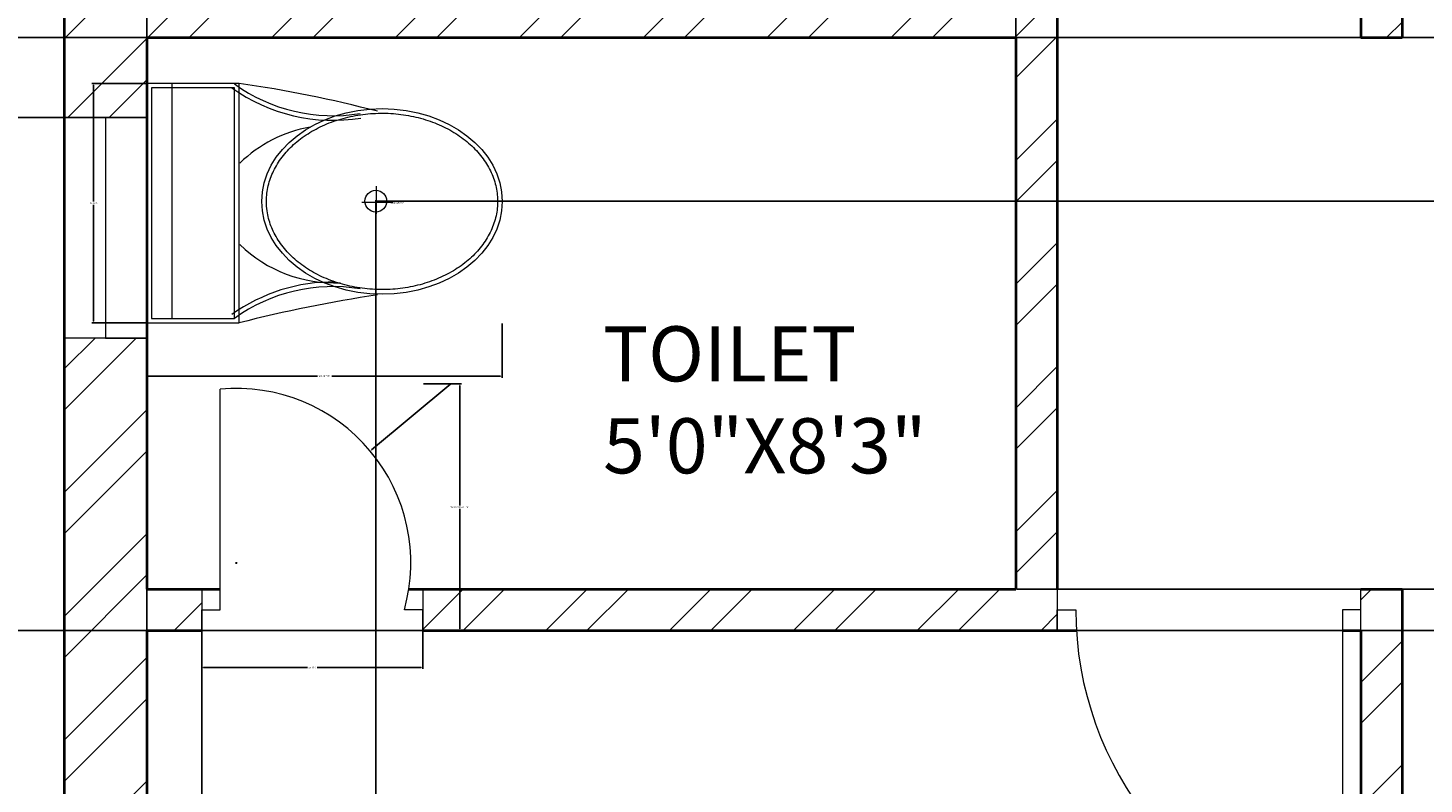
# Model space of a CAD drawing. Units: inches. Extents: x 1355 to 2746, y 1171 to 2751.
# Tile 8 of 24: x 1511 to 1663, y 1901 to 1983. Entities that reach past the tile are written whole.
import ezdxf

# ---------------------------------------------------------------- set-up
doc = ezdxf.new("R2010")
doc.units = ezdxf.units.IN
for name, color, linetype, lineweight in [('A-ANNO-DIMS', 2, 'Continuous', 18), ('A-AREA-IDEN', 7, 'Continuous', 18), ('A-DOOR', 3, 'Continuous', 20), ('A-FLOR-FIXT', 9, 'Continuous', 18), ('A-GLAZ', 4, 'Continuous', 18), ('A-WALL', 7, 'Continuous', 40), ('A-WALL-PATT', 252, 'Continuous', 13)]:
    doc.layers.add(name, color=color, linetype=linetype, lineweight=lineweight)
doc.styles.get("Standard").update_dxf_attribs({"font": 'arial.ttf'})
doc.dimstyles.get("Standard").update_dxf_attribs({"dimtxt": 0.18, "dimasz": 0.18, "dimexe": 0.18, "dimexo": 0.0625, "dimgap": 0.09, "dimtad": 0, "dimtih": 1, "dimtoh": 1, "dimdec": 4, "dimzin": 0, "dimdsep": 46, "dimtxsty": 'Standard', "dimcen": 0.09, "dimadec": 0, "dimazin": 0, "dimtfac": 1, "dimtdec": 4, "dimtofl": 0, "dimtmove": 0, "dimatfit": 3, "dimfxl": 1, "dimtolj": 1, "dimtzin": 0, "dimarcsym": 0})

# ---------------------------------------------------------------- blocks, each defined once
blk = doc.blocks.new('A$C31115884')
for p, q in [((257.5, 466.4), (257.5, 523.2)), ((283.1, 497.7), (223.4, 497.7)), ((0, 200), (0, 0)), ((520, 200), (0, 200)), ((10, 190), (10, 10)), ((510, 190), (10, 190)), ((510, 10), (510, 190)), ((520, 0), (520, 200)), ((510, 54.5), (0, 54.5)), ((10, 10), (510, 10)), ((0, 0), (520, 0))]:
    blk.add_line(p, q)
blk.add_circle((255.6, 496.4), 23.6)
for centre, radius, start, end in [((2777.7, -204.6), 2807, 165.4549, 171.7133), ((3237, 905), 2807, 188.2867, 194.5451), ((-294.5, 403.3), 364.7, 324.2091, 9.3499), ((-294.5, 403.3), 374.7, 324.2091, 9.3499), ((805.8, 403.3), 364.7, 170.6501, 215.7909), ((139.5, 406.2), 293.5, 315.8436, 2.6563), ((805.8, 403.3), 374.7, 179.2036, 215.7909), ((383.6, 406.2), 293.5, 190.2774, 224.1564)]:
    blk.add_arc(centre, radius, start, end)
blk.add_ellipse((256.2, 509.9), major_axis=(0, -260.7), ratio=0.772727)
blk.add_open_spline([(256.2, 259.2), (263.1, 259.2), (270, 259.7), (287.8, 262.3), (298.7, 265.1), (319.9, 273.1), (330.2, 278.4), (350.1, 291.1), (359.7, 298.7), (377.7, 315.9), (386.2, 325.5), (401.7, 346.6), (408.8, 358.1), (421.3, 382.5), (426.8, 395.5), (435.9, 422.4), (439.5, 436.4), (444.8, 465.1), (446.5, 479.7), (447.9, 509.2), (447.6, 524), (445, 553.3), (442.7, 567.8), (436.3, 596), (432.1, 609.7), (421.9, 636), (416, 648.6), (402.5, 672.1), (395, 683), (378.6, 703), (369.8, 712.1), (351.1, 728), (341.3, 734.8), (320.9, 746.2), (310.4, 750.7), (288.9, 757.3), (278, 759.4), (256, 761), (245, 760.6), (223.1, 757.2), (212.3, 754.3), (191.1, 746.1), (180.8, 740.7), (160.9, 727.8), (151.4, 720.1), (133.5, 702.7), (125.1, 693), (109.6, 671.7), (102.6, 660.2), (90.2, 635.7), (84.9, 622.7), (76, 595.6), (72.4, 581.6), (67.2, 552.9), (65.6, 538.2), (64.4, 508.8), (64.8, 494), (67.5, 464.7), (69.9, 450.2), (76.6, 422), (80.8, 408.3), (91.1, 382.2), (97.2, 369.7), (110.8, 346.3), (118.4, 335.4), (134.8, 315.6), (143.7, 306.7), (162.4, 290.9), (172.3, 284.2), (192.8, 273), (203.3, 268.6), (224.8, 262.2), (235.8, 260.2), (249.9, 259.3), (253, 259.2), (256.2, 259.2)], degree=3, knots=[0, 0, 0, 0, 0.110105, 0.110105, 0.285049, 0.285049, 0.459994, 0.459994, 0.634938, 0.634938, 0.809882, 0.809882, 0.984827, 0.984827, 1.159771, 1.159771, 1.334715, 1.334715, 1.50966, 1.50966, 1.684604, 1.684604, 1.859549, 1.859549, 2.034493, 2.034493, 2.209437, 2.209437, 2.384382, 2.384382, 2.559326, 2.559326, 2.73427, 2.73427, 2.909215, 2.909215, 3.084159, 3.084159, 3.259103, 3.259103, 3.434048, 3.434048, 3.608992, 3.608992, 3.783936, 3.783936, 3.958881, 3.958881, 4.133825, 4.133825, 4.30877, 4.30877, 4.483714, 4.483714, 4.658658, 4.658658, 4.833603, 4.833603, 5.008547, 5.008547, 5.183491, 5.183491, 5.358436, 5.358436, 5.53338, 5.53338, 5.708324, 5.708324, 5.883269, 5.883269, 6.058213, 6.058213, 6.233158, 6.233158, 6.283185, 6.283185, 6.283185, 6.283185])
blk = doc.blocks.new('WINDOW-PLAN-24')
for p, q in [((0, 24), (9, 24)), ((9, 24), (4.5, 24)), ((4.5, 24), (4.5, 0)), ((4.5, 0), (0, 0)), ((0, 0), (9, 0))]:
    blk.add_line(p, q)
blk = doc.blocks.new('DOOR-WC-01')
for p, q in [((2, 2.25), (2, 26.25)), ((0, 4.5), (0, 0)), ((24.04, 4.5), (24.04, 0)), ((0, 0), (0, 2.25)), ((0, 2.25), (2, 2.25)), ((24.04, 2.25), (22.04, 2.25)), ((24.04, 0), (24.04, 2.25))]:
    blk.add_line(p, q)
blk.add_arc((3.76, 7.35), 18.98, 344.4049, 95.3143)
blk = doc.blocks.new('DOOR-BEDROOM-NW')
for p, q in [((0, 38.25), (0, 33.75)), ((33, 33.75), (33, 38.25)), ((0, 33.75), (0, 36)), ((0, 36), (2, 36)), ((33, 36), (31, 36)), ((31, 36), (31, 0))]:
    blk.add_line(p, q)
blk.add_arc((38.85, 36), 36.84, 180, 257.7067)
blk = doc.blocks.new('*D35')
at = {"layer": 'A-ANNO-DIMS', "color": 0, "lineweight": -2, "transparency": 16777216}
for p, q in [((1523.71, 1950.69), (1523.71, 1944.78)), ((1562.34, 1950.69), (1562.34, 1944.78)), ((1523.89, 1944.96), (1542.25, 1944.96)), ((1562.16, 1944.96), (1543.8, 1944.96))]:
    blk.add_line(p, q, dxfattribs=at)
at = {"layer": 'A-ANNO-DIMS', "color": 0, "transparency": 16777216}
for points in [[(1523.89, 1944.99), (1523.89, 1944.93), (1523.71, 1944.96)], [(1562.16, 1944.99), (1562.16, 1944.93), (1562.34, 1944.96)]]:
    blk.add_solid(points, dxfattribs=at)
at = {"layer": 'Defpoints', "color": 0, "transparency": 16777216}
for p in [(1523.71, 1950.75), (1562.34, 1950.75), (1562.34, 1944.96)]:
    blk.add_point(p, dxfattribs=at)
at = {"layer": 'A-ANNO-DIMS', "color": 0, "transparency": 16777216, "insert": (1543.02, 1944.96), "char_height": 0.18, "attachment_point": 5}
blk.add_mtext('\\A1;WC 39 TYP.', dxfattribs=at)
blk = doc.blocks.new('*D36')
at = {"layer": 'A-ANNO-DIMS', "color": 0, "lineweight": -2, "transparency": 16777216}
for p, q in [((1523.65, 1976.82), (1517.73, 1976.82)), ((1517.91, 1976.64), (1517.91, 1963.97)), ((1517.91, 1950.93), (1517.91, 1963.61)), ((1523.65, 1950.75), (1517.73, 1950.75))]:
    blk.add_line(p, q, dxfattribs=at)
at = {"layer": 'A-ANNO-DIMS', "color": 0, "transparency": 16777216}
for points in [[(1517.88, 1976.64), (1517.94, 1976.64), (1517.91, 1976.82)], [(1517.88, 1950.93), (1517.94, 1950.93), (1517.91, 1950.75)]]:
    blk.add_solid(points, dxfattribs=at)
at = {"layer": 'Defpoints', "color": 0, "transparency": 16777216}
for p in [(1523.71, 1976.82), (1517.91, 1950.75), (1523.71, 1950.75)]:
    blk.add_point(p, dxfattribs=at)
at = {"layer": 'A-ANNO-DIMS', "color": 0, "transparency": 16777216, "insert": (1517.91, 1963.79), "char_height": 0.18, "attachment_point": 5}
blk.add_mtext('\\A1;26 TYP.', dxfattribs=at)
blk = doc.blocks.new('*D53')
at = {"layer": 'A-ANNO-DIMS', "color": 0, "lineweight": -2, "transparency": 16777216}
for p, q in [((1553.77, 1944.13), (1557.91, 1944.13)), ((1557.73, 1943.95), (1557.73, 1930.9)), ((1557.73, 1917.48), (1557.73, 1930.53)), ((1553.77, 1917.3), (1557.91, 1917.3))]:
    blk.add_line(p, q, dxfattribs=at)
at = {"layer": 'A-ANNO-DIMS', "color": 0, "transparency": 16777216}
for points in [[(1557.7, 1943.95), (1557.76, 1943.95), (1557.73, 1944.13)], [(1557.7, 1917.48), (1557.76, 1917.48), (1557.73, 1917.3)]]:
    blk.add_solid(points, dxfattribs=at)
at = {"layer": 'Defpoints', "color": 0, "transparency": 16777216}
for p in [(1553.71, 1944.13), (1557.73, 1944.13), (1553.71, 1917.3)]:
    blk.add_point(p, dxfattribs=at)
at = {"layer": 'A-ANNO-DIMS', "color": 0, "transparency": 16777216, "insert": (1557.73, 1930.72), "char_height": 0.18, "attachment_point": 5}
blk.add_mtext('\\A1;WC DOOR 27 TYP.', dxfattribs=at)
blk = doc.blocks.new('*D54')
at = {"layer": 'A-ANNO-DIMS', "color": 0, "lineweight": -2, "transparency": 16777216}
for p, q in [((1529.67, 1917.24), (1529.67, 1913.1)), ((1553.71, 1917.24), (1553.71, 1913.1)), ((1529.85, 1913.28), (1541.16, 1913.28)), ((1553.53, 1913.28), (1542.22, 1913.28))]:
    blk.add_line(p, q, dxfattribs=at)
at = {"layer": 'A-ANNO-DIMS', "color": 0, "transparency": 16777216}
for points in [[(1529.85, 1913.31), (1529.85, 1913.25), (1529.67, 1913.28)], [(1553.53, 1913.31), (1553.53, 1913.25), (1553.71, 1913.28)]]:
    blk.add_solid(points, dxfattribs=at)
at = {"layer": 'Defpoints', "color": 0, "transparency": 16777216}
for p in [(1529.67, 1917.3), (1553.71, 1917.3), (1553.71, 1913.28)]:
    blk.add_point(p, dxfattribs=at)
at = {"layer": 'A-ANNO-DIMS', "color": 0, "transparency": 16777216, "insert": (1541.69, 1913.28), "char_height": 0.18, "attachment_point": 5}
blk.add_mtext('\\A1;24 TYP.', dxfattribs=at)
blk = doc.blocks.new('*D96')
at = {"layer": 'A-ANNO-DIMS', "color": 0, "lineweight": -2, "transparency": 16777216}
for p, q in [((1514.65, 2139.3), (1407.53, 2139.3)), ((1407.71, 2139.12), (1407.71, 1725.48)), ((1407.71, 1311.48), (1407.71, 1725.12)), ((1514.65, 1311.3), (1407.53, 1311.3))]:
    blk.add_line(p, q, dxfattribs=at)
at = {"layer": 'A-ANNO-DIMS', "color": 0, "transparency": 16777216}
for points in [[(1407.68, 2139.12), (1407.74, 2139.12), (1407.71, 2139.3)], [(1407.68, 1311.48), (1407.74, 1311.48), (1407.71, 1311.3)]]:
    blk.add_solid(points, dxfattribs=at)
at = {"layer": 'Defpoints', "color": 0, "transparency": 16777216}
for p in [(1407.71, 2139.3), (1514.71, 2139.3), (1514.71, 1311.3)]:
    blk.add_point(p, dxfattribs=at)
at = {"layer": 'A-ANNO-DIMS', "color": 0, "transparency": 16777216, "insert": (1407.71, 1725.3), "char_height": 0.18, "attachment_point": 5}
blk.add_mtext('\\A1;828', dxfattribs=at)
blk = doc.blocks.new('*D103')
at = {"layer": 'A-ANNO-DIMS', "color": 0, "lineweight": -2, "transparency": 16777216}
for p, q in [((2089.33, 1917.3), (1407.53, 1917.3)), ((1407.71, 1917.12), (1407.71, 1840.98)), ((1407.71, 1764.48), (1407.71, 1840.62)), ((2089.33, 1764.3), (1407.53, 1764.3))]:
    blk.add_line(p, q, dxfattribs=at)
at = {"layer": 'A-ANNO-DIMS', "color": 0, "transparency": 16777216}
for points in [[(1407.68, 1917.12), (1407.74, 1917.12), (1407.71, 1917.3)], [(1407.68, 1764.48), (1407.74, 1764.48), (1407.71, 1764.3)]]:
    blk.add_solid(points, dxfattribs=at)
at = {"layer": 'Defpoints', "color": 0, "transparency": 16777216}
for p in [(1407.71, 1917.3), (2089.39, 1917.3), (2089.39, 1764.3)]:
    blk.add_point(p, dxfattribs=at)
at = {"layer": 'A-ANNO-DIMS', "color": 0, "transparency": 16777216, "insert": (1407.71, 1840.8), "char_height": 0.18, "attachment_point": 5}
blk.add_mtext('\\A1;153', dxfattribs=at)
blk = doc.blocks.new('*D104')
at = {"layer": 'A-ANNO-DIMS', "color": 0, "lineweight": -2, "transparency": 16777216}
for p, q in [((2089.33, 1986.3), (1407.53, 1986.3)), ((1407.71, 1986.12), (1407.71, 1951.98)), ((1407.71, 1917.48), (1407.71, 1951.62)), ((2089.33, 1917.3), (1407.53, 1917.3))]:
    blk.add_line(p, q, dxfattribs=at)
at = {"layer": 'A-ANNO-DIMS', "color": 0, "transparency": 16777216}
for points in [[(1407.68, 1986.12), (1407.74, 1986.12), (1407.71, 1986.3)], [(1407.68, 1917.48), (1407.74, 1917.48), (1407.71, 1917.3)]]:
    blk.add_solid(points, dxfattribs=at)
at = {"layer": 'Defpoints', "color": 0, "transparency": 16777216}
for p in [(1407.71, 1986.3), (2089.39, 1986.3), (2089.39, 1917.3)]:
    blk.add_point(p, dxfattribs=at)
at = {"layer": 'A-ANNO-DIMS', "color": 0, "transparency": 16777216, "insert": (1407.71, 1951.8), "char_height": 0.18, "attachment_point": 5}
blk.add_mtext('\\A1;69', dxfattribs=at)
blk = doc.blocks.new('*D135')
at = {"layer": 'A-ANNO-DIMS', "color": 0, "lineweight": -2, "transparency": 16777216}
for p, q in [((1523.71, 1981.86), (1523.71, 2716.58)), ((1523.89, 2716.4), (1570.63, 2716.4)), ((1618.03, 2716.4), (1571.28, 2716.4)), ((1618.21, 1981.86), (1618.21, 2716.58))]:
    blk.add_line(p, q, dxfattribs=at)
at = {"layer": 'A-ANNO-DIMS', "color": 0, "transparency": 16777216}
for points in [[(1523.89, 2716.43), (1523.89, 2716.37), (1523.71, 2716.4)], [(1618.03, 2716.43), (1618.03, 2716.37), (1618.21, 2716.4)]]:
    blk.add_solid(points, dxfattribs=at)
at = {"layer": 'Defpoints', "color": 0, "transparency": 16777216}
for p in [(1618.21, 2716.4), (1523.71, 1981.8), (1618.21, 1981.8)]:
    blk.add_point(p, dxfattribs=at)
at = {"layer": 'A-ANNO-DIMS', "color": 0, "transparency": 16777216, "insert": (1570.96, 2716.4), "char_height": 0.18, "attachment_point": 5}
blk.add_mtext('\\A1;94.5', dxfattribs=at)
blk = doc.blocks.new('*D136')
at = {"layer": 'A-ANNO-DIMS', "color": 0, "lineweight": -2, "transparency": 16777216}
for p, q in [((1618.27, 1981.8), (2648.07, 1981.8)), ((2647.89, 1981.62), (2647.89, 1951.98)), ((2647.89, 1921.98), (2647.89, 1951.62)), ((1618.27, 1921.8), (2648.07, 1921.8))]:
    blk.add_line(p, q, dxfattribs=at)
at = {"layer": 'A-ANNO-DIMS', "color": 0, "transparency": 16777216}
for points in [[(2647.86, 1981.62), (2647.92, 1981.62), (2647.89, 1981.8)], [(2647.86, 1921.98), (2647.92, 1921.98), (2647.89, 1921.8)]]:
    blk.add_solid(points, dxfattribs=at)
at = {"layer": 'Defpoints', "color": 0, "transparency": 16777216}
for p in [(1618.21, 1981.8), (2647.89, 1981.8), (1618.21, 1921.8)]:
    blk.add_point(p, dxfattribs=at)
at = {"layer": 'A-ANNO-DIMS', "color": 0, "transparency": 16777216, "insert": (2647.89, 1951.8), "char_height": 0.18, "attachment_point": 5}
blk.add_mtext('\\A1;60', dxfattribs=at)
blk = doc.blocks.new('*D137')
at = {"layer": 'A-ANNO-DIMS', "color": 0, "lineweight": -2, "transparency": 16777216}
for p, q in [((1523.71, 1921.74), (1523.71, 1171.06)), ((1529.67, 1919.49), (1529.67, 1171.06)), ((1523.89, 1171.24), (1526.36, 1171.24)), ((1529.49, 1171.24), (1527.01, 1171.24))]:
    blk.add_line(p, q, dxfattribs=at)
at = {"layer": 'A-ANNO-DIMS', "color": 0, "transparency": 16777216}
for points in [[(1523.89, 1171.27), (1523.89, 1171.21), (1523.71, 1171.24)], [(1529.49, 1171.27), (1529.49, 1171.21), (1529.67, 1171.24)]]:
    blk.add_solid(points, dxfattribs=at)
at = {"layer": 'Defpoints', "color": 0, "transparency": 16777216}
for p in [(1523.71, 1921.8), (1529.67, 1919.55), (1529.67, 1171.24)]:
    blk.add_point(p, dxfattribs=at)
at = {"layer": 'A-ANNO-DIMS', "color": 0, "transparency": 16777216, "insert": (1526.69, 1171.24), "char_height": 0.18, "attachment_point": 5}
blk.add_mtext('\\A1;5.96', dxfattribs=at)
blk = doc.blocks.new('*D138')
at = {"layer": 'A-ANNO-DIMS', "color": 0, "lineweight": -2, "transparency": 16777216}
for p, q in [((1523.65, 1981.8), (1407.53, 1981.8)), ((1407.71, 1981.62), (1407.71, 1977.64)), ((1407.71, 1973.29), (1407.71, 1977.28)), ((1523.65, 1973.11), (1407.53, 1973.11))]:
    blk.add_line(p, q, dxfattribs=at)
at = {"layer": 'A-ANNO-DIMS', "color": 0, "transparency": 16777216}
for points in [[(1407.68, 1981.62), (1407.74, 1981.62), (1407.71, 1981.8)], [(1407.68, 1973.29), (1407.74, 1973.29), (1407.71, 1973.11)]]:
    blk.add_solid(points, dxfattribs=at)
at = {"layer": 'Defpoints', "color": 0, "transparency": 16777216}
for p in [(1407.71, 1981.8), (1523.71, 1981.8), (1523.71, 1973.11)]:
    blk.add_point(p, dxfattribs=at)
at = {"layer": 'A-ANNO-DIMS', "color": 0, "transparency": 16777216, "insert": (1407.71, 1977.46), "char_height": 0.18, "attachment_point": 5}
blk.add_mtext('\\A1;8.688', dxfattribs=at)
blk = doc.blocks.new('*D139')
at = {"layer": 'A-ANNO-DIMS', "color": 0, "lineweight": -2, "transparency": 16777216}
for p, q in [((1523.77, 1981.8), (2648.07, 1981.8)), ((2647.89, 1981.62), (2647.89, 1973.09)), ((2647.89, 1964.19), (2647.89, 1972.72)), ((1548.66, 1964.01), (2648.07, 1964.01))]:
    blk.add_line(p, q, dxfattribs=at)
at = {"layer": 'A-ANNO-DIMS', "color": 0, "transparency": 16777216}
for points in [[(2647.86, 1981.62), (2647.92, 1981.62), (2647.89, 1981.8)], [(2647.86, 1964.19), (2647.92, 1964.19), (2647.89, 1964.01)]]:
    blk.add_solid(points, dxfattribs=at)
at = {"layer": 'Defpoints', "color": 0, "transparency": 16777216}
for p in [(1523.71, 1981.8), (1548.6, 1964.01), (2647.89, 1964.01)]:
    blk.add_point(p, dxfattribs=at)
at = {"layer": 'A-ANNO-DIMS', "color": 0, "transparency": 16777216, "insert": (2647.89, 1972.9), "char_height": 0.18, "attachment_point": 5}
blk.add_mtext('\\A1;17.795', dxfattribs=at)
blk = doc.blocks.new('*D140')
at = {"layer": 'A-ANNO-DIMS', "color": 0, "lineweight": -2, "transparency": 16777216}
for p, q in [((1523.71, 1973.05), (1523.71, 1171.06)), ((1548.6, 1963.94), (1548.6, 1171.06)), ((1523.89, 1171.24), (1535.76, 1171.24)), ((1548.42, 1171.24), (1536.55, 1171.24))]:
    blk.add_line(p, q, dxfattribs=at)
at = {"layer": 'A-ANNO-DIMS', "color": 0, "transparency": 16777216}
for points in [[(1523.89, 1171.27), (1523.89, 1171.21), (1523.71, 1171.24)], [(1548.42, 1171.27), (1548.42, 1171.21), (1548.6, 1171.24)]]:
    blk.add_solid(points, dxfattribs=at)
at = {"layer": 'Defpoints', "color": 0, "transparency": 16777216}
for p in [(1523.71, 1973.11), (1548.6, 1964.01), (1548.6, 1171.24)]:
    blk.add_point(p, dxfattribs=at)
at = {"layer": 'A-ANNO-DIMS', "color": 0, "transparency": 16777216, "insert": (1536.15, 1171.24), "char_height": 0.18, "attachment_point": 5}
blk.add_mtext('\\A1;24.89', dxfattribs=at)
blk = doc.blocks.new('*D148')
at = {"layer": 'A-ANNO-DIMS', "color": 0, "lineweight": -2, "transparency": 16777216}
for p, q in [((1548.51, 1964.01), (1548.69, 1964.01)), ((1548.6, 1963.92), (1548.6, 1964.1)), ((1550.48, 1963.82), (1549.95, 1963.88))]:
    blk.add_line(p, q, dxfattribs=at)
at = {"layer": 'A-ANNO-DIMS', "color": 0, "transparency": 16777216}
blk.add_solid([(1549.96, 1963.91), (1549.95, 1963.85), (1549.78, 1963.89)], dxfattribs=at)
at = {"layer": 'Defpoints', "color": 0, "transparency": 16777216}
for p in [(1547.42, 1964.12), (1549.78, 1963.89)]:
    blk.add_point(p, dxfattribs=at)
at = {"layer": 'A-ANNO-DIMS', "color": 0, "transparency": 16777216, "insert": (1551.1, 1963.82), "char_height": 0.18, "attachment_point": 5}
blk.add_mtext('\\A1;4X ∅2.37', dxfattribs=at)
blk = doc.blocks.new('*D150')
at = {"layer": 'A-ANNO-DIMS', "color": 0, "lineweight": -2, "transparency": 16777216}
for p, q in [((1556.74, 1944.12), (1548.13, 1936.93)), ((1556.92, 1944.12), (1556.74, 1944.12)), ((1533.34, 1924.65), (1533.52, 1924.65)), ((1533.43, 1924.56), (1533.43, 1924.74))]:
    blk.add_line(p, q, dxfattribs=at)
at = {"layer": 'A-ANNO-DIMS', "color": 0, "transparency": 16777216}
blk.add_solid([(1548.11, 1936.96), (1548.15, 1936.91), (1548, 1936.82)], dxfattribs=at)
at = {"layer": 'Defpoints', "color": 0, "transparency": 16777216}
for p in [(1548, 1936.82), (1533.43, 1924.65)]:
    blk.add_point(p, dxfattribs=at)
at = {"layer": 'A-ANNO-DIMS', "color": 0, "transparency": 16777216, "insert": (1557.4, 1944.12), "char_height": 0.18, "attachment_point": 5}
blk.add_mtext('\\A1;R18.98', dxfattribs=at)

msp = doc.modelspace()

# ---------------------------------------------------------------- hatches: boundary and pattern name
at = {"layer": 'A-WALL-PATT'}
h = msp.add_hatch(dxfattribs=at)
h.set_pattern_fill('ANSI32', color=256)
h.paths.add_polyline_path([(1660.2083, 2139.3018), (1614.5977, 2139.3018), (1614.5977, 2130.3018), (1655.7083, 2130.3018), (1655.7083, 1981.8018), (1660.2083, 1981.8018), (1660.2083, 2090.7225), (1692.5832, 2090.7225), (1692.5832, 2095.2225), (1660.2083, 2095.2225)])
h.paths.add_polyline_path([(1523.7083, 2130.3018), (1554.5977, 2130.3018), (1554.5977, 2134.8018), (1554.5977, 2139.3018), (1514.7083, 2139.3018), (1514.7083, 2071.8385), (1523.7083, 2071.8385)])
h.paths.add_polyline_path([(1940.7083, 2139.3018), (1883.7928, 2139.3018), (1883.7928, 2130.3018), (1931.7083, 2130.3018), (1931.7083, 2098.3333), (1940.7083, 2098.3333)])
h.paths.add_polyline_path([(1799.7083, 2130.3018), (1823.7928, 2130.3018), (1823.7928, 2134.8018), (1823.7928, 2139.3018), (1795.2083, 2139.3018), (1795.2083, 2130.3018), (1795.2083, 2095.2225), (1759.2134, 2095.2225), (1759.2134, 2090.7225), (1795.2083, 2090.7225), (1795.2083, 1981.8018), (1799.7083, 1981.8018), (1799.7083, 1986.3018)])
h.paths.add_polyline_path([(1940.7083, 2038.3333), (1931.7083, 2038.3333), (1931.7083, 1986.3018), (1832.7083, 1986.3018), (1832.7083, 1947.1338), (1837.2083, 1947.1338), (1837.2083, 1981.8018), (1931.7083, 1981.8018), (1931.7083, 1967.1939), (1940.7083, 1967.1939)])
h.paths.add_polyline_path([(1940.7083, 1943.1939), (1931.7083, 1943.1939), (1931.7083, 1921.8018), (1837.2083, 1921.8018), (1837.2083, 1926.0511), (1832.7083, 1926.0511), (1832.7083, 1917.3018), (1931.7083, 1917.3018), (1931.7083, 1908.3321), (1940.7083, 1908.3321)])
h.paths.add_polyline_path([(1940.7083, 1884.3321), (1931.7083, 1884.3321), (1931.7083, 1869.3018), (1899.4583, 1869.3018), (1899.4583, 1864.8018), (1931.7083, 1864.8018), (1931.7083, 1773.3018), (1786.5143, 1773.3018), (1786.5143, 1764.3018), (1844.7083, 1764.3018), (1844.7083, 1748.9343), (1853.7083, 1748.9343), (1853.7083, 1764.3018), (1931.7083, 1764.3018), (1931.7083, 1652.9424), (1940.7083, 1652.9424)])
h.paths.add_polyline_path([(1799.7083, 1864.8018), (1806.0522, 1864.8018), (1806.0522, 1867.0518), (1806.0522, 1869.3018), (1799.7083, 1869.3018), (1799.7083, 1917.3018), (1799.7083, 1921.8018), (1795.2083, 1921.8018), (1795.2083, 1773.3018), (1799.7083, 1773.3018)])
h.paths.add_polyline_path([(1872.8988, 1867.0518), (1872.8988, 1869.3018), (1867.2083, 1869.3018), (1867.2083, 1917.3018), (1862.7083, 1917.3018), (1862.7083, 1869.3018), (1836.9546, 1869.3018), (1836.9546, 1864.8018), (1862.7083, 1864.8018), (1872.8988, 1864.8018)])
h.paths.add_polyline_path([(1749.2197, 1773.3018), (1655.7083, 1773.3018), (1523.7083, 1773.3018), (1523.7083, 1828.4963), (1514.7083, 1828.4963), (1514.7083, 1753.9033), (1519.2083, 1753.9033), (1523.7083, 1753.9033), (1523.7083, 1764.3018), (1655.7083, 1764.3018), (1749.2197, 1764.3018), (1749.2197, 1768.8018)])
h.paths.add_polyline_path([(1660.2083, 1921.8018), (1655.7083, 1921.8018), (1655.7083, 1917.3018), (1655.7083, 1773.3018), (1660.2083, 1773.3018)])
h.paths.add_polyline_path([(1523.7083, 2011.8385), (1514.7083, 2011.8385), (1514.7083, 1973.114), (1519.2083, 1973.114), (1523.7083, 1973.114), (1523.7083, 1976.8227), (1523.7083, 1981.8018), (1618.2083, 1981.8018), (1618.2083, 1921.8018), (1553.707, 1921.8018), (1553.707, 1917.3018), (1622.7083, 1917.3018), (1622.7083, 1919.5518), (1622.7083, 1921.8018), (1622.7083, 1986.3018), (1523.7083, 1986.3018)])
h.paths.add_polyline_path([(1529.6686, 1919.5518), (1529.6686, 1921.8018), (1523.7083, 1921.8018), (1523.7083, 1949.114), (1514.7083, 1949.114), (1514.7083, 1888.4963), (1523.7083, 1888.4963), (1523.7083, 1917.3018), (1529.6686, 1917.3018)])
h.paths.add_polyline_path([(1538.9419, 1775.643), (1585.5504, 1775.643), (1585.5504, 1798.0318), (1538.9419, 1798.0318)], flags=25)
h.paths.add_polyline_path([(1696.7097, 1497.3356), (1769.5651, 1497.3356), (1769.5651, 1523.4559), (1696.7097, 1523.4559)], flags=9)
h.paths.add_polyline_path([(1629.1643, 1230.5133), (1877.0879, 1230.5133), (1877.0879, 1267.606), (1629.1643, 1267.606)], flags=9)
h.paths.add_polyline_path([(2533.4462, 2215.4033), (2579.9292, 2215.4033), (2579.9292, 2231.889), (2533.4462, 2231.889)], flags=9)
h.paths.add_polyline_path([(2540.822, 2515.6945), (2594.2245, 2515.6945), (2594.2245, 2545.5463), (2540.822, 2545.5463)], flags=9)
h.paths.add_polyline_path([(2535.9857, 2588.2819), (2582.4687, 2588.2819), (2582.4687, 2604.7675), (2535.9857, 2604.7675)], flags=9)
h.paths.add_polyline_path([(2537.1627, 2617.1172), (2649.1245, 2617.1172), (2649.1245, 2633.6029), (2537.1627, 2633.6029)], flags=9)
h.paths.add_polyline_path([(2218.0051, 2168.228), (2363.9573, 2168.228), (2363.9573, 2205.3208), (2218.0051, 2205.3208)], flags=9)
h.paths.add_polyline_path([(1650.2156, 2165.3631), (1800.3547, 2165.3631), (1800.3547, 2202.4559), (1650.2156, 2202.4559)], flags=9)
h.paths.add_polyline_path([(2553.9592, 1610.7663), (2588.4203, 1610.7663), (2588.4203, 1660.2233), (2553.9592, 1660.2233)], flags=9)
h.paths.add_polyline_path([(1549.0868, 1648.2033), (1595.6952, 1648.2033), (1595.6952, 1670.5921), (1549.0868, 1670.5921)], flags=9)
h.paths.add_polyline_path([(1546.9525, 1502.0931), (1583.3413, 1502.0931), (1583.3413, 1524.4819), (1546.9525, 1524.4819)], flags=9)
h.paths.add_polyline_path([(1540.7704, 1433.4431), (1587.3788, 1433.4431), (1587.3788, 1455.8319), (1540.7704, 1455.8319)], flags=9)
h.paths.add_polyline_path([(1683.6524, 1321.5269), (1760.6169, 1321.5269), (1760.6169, 1333.8911), (1683.6524, 1333.8911)], flags=9)
h.paths.add_polyline_path([(1832.0485, 1356.0874), (1873.0989, 1356.0874), (1873.0989, 1378.4762), (1832.0485, 1378.4762)], flags=9)
h.paths.add_polyline_path([(1877.9694, 1431.2138), (1926.3827, 1431.2138), (1926.3827, 1453.578), (1877.9694, 1453.578)], flags=9)
h.paths.add_polyline_path([(1847.3106, 1499.8371), (1883.6994, 1499.8371), (1883.6994, 1522.2259), (1847.3106, 1522.2259)], flags=9)
h.paths.add_polyline_path([(1813.7015, 1640.7287), (1860.3099, 1640.7287), (1860.3099, 1663.1175), (1813.7015, 1663.1175)], flags=9)
h.paths.add_polyline_path([(1876.2576, 1710.2471), (1912.9452, 1710.2471), (1912.9452, 1732.6359), (1876.2576, 1732.6359)], flags=25)
h.paths.add_polyline_path([(1695.9163, 1715.3064), (1736.9668, 1715.3064), (1736.9668, 1737.6952), (1695.9163, 1737.6952)], flags=9)
h.paths.add_polyline_path([(1881.8583, 1888.9094), (1930.2717, 1888.9094), (1930.2717, 1911.2737), (1881.8583, 1911.2737)], flags=9)
h.paths.add_polyline_path([(1823.9298, 1798.6431), (1864.9803, 1798.6431), (1864.9803, 1821.0319), (1823.9298, 1821.0319)], flags=25)
h.paths.add_polyline_path([(1845.6062, 1948.1408), (1881.995, 1948.1408), (1881.995, 1970.5296), (1845.6062, 1970.5296)], flags=25)
h.paths.add_polyline_path([(1849.027, 1991.5151), (1895.6355, 1991.5151), (1895.6355, 2013.9039), (1849.027, 2013.9039)], flags=25)
h.paths.add_polyline_path([(1684.9725, 2113.8416), (1764.2658, 2113.8416), (1764.2658, 2126.2058), (1684.9725, 2126.2058)], flags=9)
h.paths.add_polyline_path([(1688.6193, 1913.0676), (1776.2005, 1913.0676), (1776.2005, 1935.4564), (1688.6193, 1935.4564)], flags=9)
h.paths.add_polyline_path([(1571.4689, 1930.9816), (1607.8577, 1930.9816), (1607.8577, 1953.3704), (1571.4689, 1953.3704)], flags=25)
h.paths.add_polyline_path([(1535.3581, 1998.3125), (1581.9665, 1998.3125), (1581.9665, 2020.7014), (1535.3581, 2020.7014)], flags=9)
h = msp.add_hatch(dxfattribs=at)
h.set_pattern_fill('ANSI32', color=256)
h.paths.add_polyline_path([(1749.2197, 1686.3018), (1732.6892, 1686.3018), (1523.7083, 1686.3018), (1523.7083, 1705.9033), (1514.7083, 1705.9033), (1514.7083, 1647.8732), (1519.2083, 1647.8732), (1523.7083, 1647.8732), (1523.7083, 1677.3018), (1655.7083, 1677.3018), (1655.7083, 1528.8018), (1660.2083, 1528.8018), (1660.2083, 1677.3018), (1732.6892, 1677.3018), (1749.2197, 1677.3018)])
h.paths.add_polyline_path([(1931.7083, 1686.3018), (1853.7083, 1686.3018), (1853.7083, 1703.5696), (1844.7083, 1703.5696), (1844.7083, 1686.3018), (1788.0274, 1686.3018), (1788.0274, 1677.3018), (1795.2083, 1677.3018), (1795.2083, 1528.8018), (1799.7083, 1528.8018), (1799.7083, 1677.3018), (1844.7083, 1677.3018), (1931.7083, 1677.3018)])
h.paths.add_polyline_path([(1931.7083, 1533.3018), (1844.7083, 1533.3018), (1832.7083, 1533.3018), (1832.7083, 1531.0518), (1832.7083, 1528.8018), (1832.7083, 1495.7519), (1837.2083, 1495.7519), (1837.2083, 1528.8018), (1931.7083, 1528.8018)])
h.paths.add_polyline_path([(1940.7083, 1592.9424), (1931.7083, 1592.9424), (1931.7083, 1506.7845), (1940.7083, 1506.7845)])
h.paths.add_polyline_path([(1940.7083, 1482.7845), (1936.2083, 1482.7845), (1931.7083, 1482.7845), (1931.7083, 1320.3018), (1880.7083, 1320.3018), (1880.7083, 1311.3018), (1940.7083, 1311.3018)])
h.paths.add_polyline_path([(1931.7083, 1468.8018), (1844.7083, 1468.8018), (1837.2083, 1468.8018), (1837.2083, 1474.34), (1832.7083, 1474.34), (1832.7083, 1468.8018), (1832.7083, 1464.3018), (1844.7083, 1464.3018), (1931.7083, 1464.3018)])
h.paths.add_polyline_path([(1863.8571, 1464.3018), (1859.3571, 1464.3018), (1859.3571, 1404.1662), (1838.1542, 1404.1662), (1838.1542, 1399.8018), (1869.4185, 1399.8018), (1869.4185, 1402.0518), (1869.4185, 1404.3018), (1863.8571, 1404.3018)])
h.paths.add_polyline_path([(1799.7083, 1399.6662), (1805.4082, 1399.6662), (1805.4082, 1401.9162), (1805.4082, 1404.1662), (1799.7083, 1404.1662), (1799.7083, 1464.3018), (1799.7083, 1468.8018), (1795.2083, 1468.8018), (1795.2083, 1356.2098), (1761.2597, 1356.2098), (1761.2597, 1351.7098), (1795.2083, 1351.7098), (1795.2083, 1320.3018), (1795.2083, 1311.3018), (1844.7083, 1311.3018), (1844.7083, 1315.8018), (1844.7083, 1320.3018), (1799.7083, 1320.3018)])
h.paths.add_polyline_path([(1692.9218, 1356.2098), (1660.2083, 1356.2098), (1660.2083, 1430.786), (1657.9583, 1430.786), (1655.7083, 1430.786), (1655.7083, 1320.3018), (1611.934, 1320.3018), (1611.934, 1311.3018), (1660.2083, 1311.3018), (1660.2083, 1351.7098), (1692.9218, 1351.7098)])
h.paths.add_polyline_path([(1523.7083, 1372.653), (1514.7083, 1372.653), (1514.7083, 1311.3018), (1551.934, 1311.3018), (1551.934, 1315.8018), (1551.934, 1320.3018), (1523.7083, 1320.3018)])
h.paths.add_polyline_path([(1523.7083, 1490.9023), (1514.7083, 1490.9023), (1514.7083, 1432.653), (1519.2083, 1432.653), (1523.7083, 1432.653)])
h.paths.add_polyline_path([(1660.2083, 1468.8018), (1622.7083, 1468.8018), (1622.7083, 1473.1566), (1618.2083, 1473.1566), (1618.2083, 1468.8018), (1523.7083, 1468.8018), (1523.7083, 1464.3018), (1655.7083, 1464.3018), (1655.7083, 1460.5634), (1660.2083, 1460.5634)])
h.paths.add_polyline_path([(1523.7083, 1587.8732), (1514.7083, 1587.8732), (1514.7083, 1514.9023), (1519.2083, 1514.9023), (1523.7083, 1514.9023)])
h.paths.add_polyline_path([(1622.7083, 1533.3018), (1523.7083, 1533.3018), (1523.7083, 1528.8018), (1618.2083, 1528.8018), (1618.2083, 1494.4205), (1622.7083, 1494.4205), (1622.7083, 1528.8018)])
h.paths.add_polyline_path([(1696.7097, 1497.3356), (1769.5651, 1497.3356), (1769.5651, 1523.4559), (1696.7097, 1523.4559)], flags=9)
h.paths.add_polyline_path([(1629.1643, 1230.5133), (1877.0879, 1230.5133), (1877.0879, 1267.606), (1629.1643, 1267.606)], flags=9)
h.paths.add_polyline_path([(2533.4462, 2215.4033), (2579.9292, 2215.4033), (2579.9292, 2231.889), (2533.4462, 2231.889)], flags=9)
h.paths.add_polyline_path([(2540.822, 2515.6945), (2594.2245, 2515.6945), (2594.2245, 2545.5463), (2540.822, 2545.5463)], flags=9)
h.paths.add_polyline_path([(2535.9857, 2588.2819), (2582.4687, 2588.2819), (2582.4687, 2604.7675), (2535.9857, 2604.7675)], flags=9)
h.paths.add_polyline_path([(2537.1627, 2617.1172), (2649.1245, 2617.1172), (2649.1245, 2633.6029), (2537.1627, 2633.6029)], flags=9)
h.paths.add_polyline_path([(2218.0051, 2168.228), (2363.9573, 2168.228), (2363.9573, 2205.3208), (2218.0051, 2205.3208)], flags=9)
h.paths.add_polyline_path([(1650.2156, 2165.3631), (1800.3547, 2165.3631), (1800.3547, 2202.4559), (1650.2156, 2202.4559)], flags=9)
h.paths.add_polyline_path([(2553.9592, 1610.7663), (2588.4203, 1610.7663), (2588.4203, 1660.2233), (2553.9592, 1660.2233)], flags=9)
h.paths.add_polyline_path([(1549.0868, 1648.2033), (1595.6952, 1648.2033), (1595.6952, 1670.5921), (1549.0868, 1670.5921)], flags=25)
h.paths.add_polyline_path([(1546.9525, 1502.0931), (1583.3413, 1502.0931), (1583.3413, 1524.4819), (1546.9525, 1524.4819)], flags=25)
h.paths.add_polyline_path([(1540.7704, 1433.4431), (1587.3788, 1433.4431), (1587.3788, 1455.8319), (1540.7704, 1455.8319)], flags=9)
h.paths.add_polyline_path([(1683.6524, 1321.5269), (1760.6169, 1321.5269), (1760.6169, 1333.8911), (1683.6524, 1333.8911)], flags=9)
h.paths.add_polyline_path([(1832.0485, 1356.0874), (1873.0989, 1356.0874), (1873.0989, 1378.4762), (1832.0485, 1378.4762)], flags=9)
h.paths.add_polyline_path([(1877.9694, 1431.2138), (1926.3827, 1431.2138), (1926.3827, 1453.578), (1877.9694, 1453.578)], flags=9)
h.paths.add_polyline_path([(1847.3106, 1499.8371), (1883.6994, 1499.8371), (1883.6994, 1522.2259), (1847.3106, 1522.2259)], flags=25)
h.paths.add_polyline_path([(1813.7015, 1640.7287), (1860.3099, 1640.7287), (1860.3099, 1663.1175), (1813.7015, 1663.1175)], flags=25)
h.paths.add_polyline_path([(1876.2576, 1710.2471), (1912.9452, 1710.2471), (1912.9452, 1732.6359), (1876.2576, 1732.6359)], flags=9)
h.paths.add_polyline_path([(1695.9163, 1715.3064), (1736.9668, 1715.3064), (1736.9668, 1737.6952), (1695.9163, 1737.6952)], flags=9)
h.paths.add_polyline_path([(1881.8583, 1888.9094), (1930.2717, 1888.9094), (1930.2717, 1911.2737), (1881.8583, 1911.2737)], flags=9)
h.paths.add_polyline_path([(1823.9298, 1798.6431), (1864.9803, 1798.6431), (1864.9803, 1821.0319), (1823.9298, 1821.0319)], flags=9)
h.paths.add_polyline_path([(1845.6062, 1948.1408), (1881.995, 1948.1408), (1881.995, 1970.5296), (1845.6062, 1970.5296)], flags=9)
h.paths.add_polyline_path([(1849.027, 1991.5151), (1895.6355, 1991.5151), (1895.6355, 2013.9039), (1849.027, 2013.9039)], flags=9)
h.paths.add_polyline_path([(1684.9725, 2113.8416), (1764.2658, 2113.8416), (1764.2658, 2126.2058), (1684.9725, 2126.2058)], flags=9)
h.paths.add_polyline_path([(1688.6193, 1913.0676), (1776.2005, 1913.0676), (1776.2005, 1935.4564), (1688.6193, 1935.4564)], flags=9)
h.paths.add_polyline_path([(1538.9419, 1775.643), (1585.5504, 1775.643), (1585.5504, 1798.0318), (1538.9419, 1798.0318)], flags=9)
h.paths.add_polyline_path([(1571.4689, 1930.9816), (1607.8577, 1930.9816), (1607.8577, 1953.3704), (1571.4689, 1953.3704)], flags=9)
h.paths.add_polyline_path([(1535.3581, 1998.3125), (1581.9665, 1998.3125), (1581.9665, 2020.7014), (1535.3581, 2020.7014)], flags=9)

# ---------------------------------------------------------------- linework, layer by layer
at = {"layer": 'A-WALL'}
for p, q in [((1514.7083, 2139.3018), (1514.7083, 1311.3018)), ((1655.7083, 2130.3018), (1655.7083, 1981.8018)), ((1660.2083, 2090.7225), (1660.2083, 1981.8018)), ((1622.7083, 1986.3018), (1622.7083, 1921.8018)), ((1523.7083, 1981.8018), (1618.2083, 1981.8018)), ((1523.7083, 1981.8018), (1523.7083, 1921.8018)), ((1618.2083, 1981.8018), (1618.2083, 1921.8018)), ((1655.7083, 1981.8018), (1660.2083, 1981.8018)), ((1523.7083, 1921.8018), (1531.6686, 1921.8018)), ((1552.1902, 1921.8018), (1618.2083, 1921.8018)), ((1655.7083, 1921.8018), (1660.2083, 1921.8018)), ((1660.2083, 1921.8018), (1660.2083, 1773.3018)), ((1523.7083, 1917.3018), (1529.6686, 1917.3018)), ((1523.7083, 1917.3018), (1523.7083, 1773.3018)), ((1553.707, 1917.3018), (1624.7771, 1917.3018)), ((1653.7083, 1917.3018), (1655.7083, 1917.3018)), ((1655.7083, 1917.3018), (1655.7083, 1773.3018))]:
    msp.add_line(p, q, dxfattribs=at)

# ---------------------------------------------------------------- block references
at = {"layer": 'A-DOOR'}
for name, p in [('DOOR-WC-01', (1529.669, 1917.302)), ('DOOR-BEDROOM-NW', (1622.708, 1883.552))]:
    msp.add_blockref(name, p, dxfattribs=at)
at = {"layer": 'A-FLOR-FIXT', "xscale": 0.0501345278177945, "yscale": 0.0501345278177945, "zscale": 0.0501345278177945, "rotation": 270}
msp.add_blockref('A$C31115884', (1523.7083, 1976.8227), dxfattribs=at)
at = {"layer": 'A-GLAZ', "extrusion": (0, 0, -1), "zscale": -1}
msp.add_blockref('WINDOW-PLAN-24', (-1523.708, 1949.114), dxfattribs=at)

# ---------------------------------------------------------------- texts
at = {"layer": 'A-AREA-IDEN', "insert": (1573.3168, 1950.3888), "char_height": 6, "attachment_point": 1}
msp.add_mtext_dynamic_manual_height_columns('TOILET\\P5\'0"X8\'3"', width=103.880443, gutter_width=12.5, heights=[0], dxfattribs=at)

# ---------------------------------------------------------------- dimensions: what is measured, and where the dimension line sits
at = {"layer": 'A-ANNO-DIMS'}
for base, p1, p2, override, picture, middle in [((1618.2083, 2716.3999), (1523.7083, 1981.8018), (1618.2083, 1981.8018), {"dimdec": 1, "dimlfac": 1, "dimrnd": 0, "dimzin": 0, "dimdsep": 46, "dimlunit": 2}, '*D135', (1570.9583, 2716.3999)), ((1548.5973, 1171.2388), (1523.7077, 1973.1139), (1548.5973, 1964.0069), {"dimdec": 2, "dimlfac": 1, "dimrnd": 0, "dimzin": 0, "dimdsep": 46, "dimlunit": 2}, '*D140', (1536.1525, 1171.2388)), ((1529.6686, 1171.2388), (1523.7083, 1921.8018), (1529.6686, 1919.5518), {"dimdec": 2, "dimlfac": 1, "dimrnd": 0, "dimzin": 0, "dimdsep": 46, "dimlunit": 2}, '*D137', (1526.6885, 1171.2388))]:
    dim = msp.add_linear_dim(base=base, p1=p1, p2=p2, dimstyle='Standard', override=override, dxfattribs=at)
    dim.commit()
    dim.dimension.update_dxf_attribs({"geometry": picture, "text_midpoint": middle})
for base, p1, p2, override, picture, middle in [((1407.7083, 2139.3018), (1514.7083, 1311.3018), (1514.7083, 2139.3018), {"dimdec": 0, "dimlfac": 1, "dimrnd": 0, "dimzin": 0, "dimdsep": 46, "dimlunit": 2}, '*D96', (1407.7083, 1725.3018)), ((1407.7083, 1986.3018), (2089.3909, 1917.3018), (2089.3909, 1986.3018), {"dimdec": 0, "dimlfac": 1, "dimrnd": 0, "dimzin": 0, "dimdsep": 46, "dimlunit": 2}, '*D104', (1407.7083, 1951.8018)), ((1407.7083, 1981.8018), (1523.7077, 1973.1139), (1523.7083, 1981.8018), {"dimdec": 3, "dimlfac": 1, "dimrnd": 0, "dimzin": 0, "dimdsep": 46, "dimlunit": 2}, '*D138', (1407.7083, 1977.4578)), ((2647.886, 1964.0069), (1523.7083, 1981.8018), (1548.5973, 1964.0069), {"dimdec": 3, "dimlfac": 1, "dimrnd": 0, "dimzin": 0, "dimdsep": 46, "dimlunit": 2}, '*D139', (2647.886, 1972.9044)), ((2647.886, 1981.8018), (1618.2083, 1921.8018), (1618.2083, 1981.8018), {"dimdec": 0, "dimlfac": 1, "dimrnd": 0, "dimzin": 0, "dimdsep": 46, "dimlunit": 2}, '*D136', (2647.886, 1951.8018)), ((1407.7083, 1917.3018), (2089.3909, 1764.3018), (2089.3909, 1917.3018), {"dimdec": 0, "dimlfac": 1, "dimrnd": 0, "dimzin": 0, "dimdsep": 46, "dimlunit": 2}, '*D103', (1407.7083, 1840.8018))]:
    dim = msp.add_linear_dim(base=base, p1=p1, p2=p2, angle=90, dimstyle='Standard', override=override, dxfattribs=at)
    dim.commit()
    dim.dimension.update_dxf_attribs({"geometry": picture, "text_midpoint": middle})
for base, p1, p2, angle, text, picture, middle in [((1517.9135, 1950.7527), (1523.7083, 1976.8227), (1523.7083, 1950.7527), 270, '<> TYP.', '*D36', (1517.9135, 1963.7877)), ((1557.7313, 1944.1303), (1553.707, 1917.3018), (1553.707, 1944.1303), 90, 'WC DOOR <> TYP.', '*D53', (1557.7313, 1930.7161))]:
    dim = msp.add_linear_dim(base=base, p1=p1, p2=p2, angle=angle, text=text, dimstyle='Standard', override={"dimdec": 0, "dimlfac": 1, "dimrnd": 0, "dimzin": 0, "dimdsep": 46, "dimlunit": 2}, dxfattribs=at)
    dim.commit()
    dim.dimension.update_dxf_attribs({"geometry": picture, "text_midpoint": middle})
dim = msp.add_diameter_dim_2p(p1=(1547.4195, 1964.121), p2=(1549.7752, 1963.8927), text='4X <>', dimstyle='Standard', override={"dimdec": 2, "dimlfac": 1, "dimrnd": 0, "dimzin": 0, "dimdsep": 46, "dimlunit": 2}, dxfattribs=at)
dim.commit()
dim.dimension.update_dxf_attribs({"geometry": '*D148', "text_midpoint": (1550.4818, 1963.8242), "dimtype": 163})
for base, p1, p2, text, picture, middle in [((1562.3405, 1944.9579), (1523.7083, 1950.7527), (1562.3405, 1950.7527), 'WC <> TYP.', '*D35', (1543.0244, 1944.9579)), ((1553.707, 1913.2776), (1529.6686, 1917.3018), (1553.707, 1917.3018), '<> TYP.', '*D54', (1541.6878, 1913.2776))]:
    dim = msp.add_linear_dim(base=base, p1=p1, p2=p2, text=text, dimstyle='Standard', override={"dimdec": 0, "dimlfac": 1, "dimrnd": 0, "dimzin": 0, "dimdsep": 46, "dimlunit": 2}, dxfattribs=at)
    dim.commit()
    dim.dimension.update_dxf_attribs({"geometry": picture, "text_midpoint": middle})
dim = msp.add_radius_dim(center=(1533.4265, 1924.6542), mpoint=(1547.9952, 1936.8182), dimstyle='Standard', override={"dimdec": 2, "dimlfac": 1, "dimrnd": 0, "dimzin": 0, "dimdsep": 46, "dimlunit": 2}, dxfattribs=at)
dim.commit()
dim.dimension.update_dxf_attribs({"geometry": '*D150', "text_midpoint": (1557.3965, 1944.1166), "dimtype": 164})

doc.saveas('drawing.dxf')
